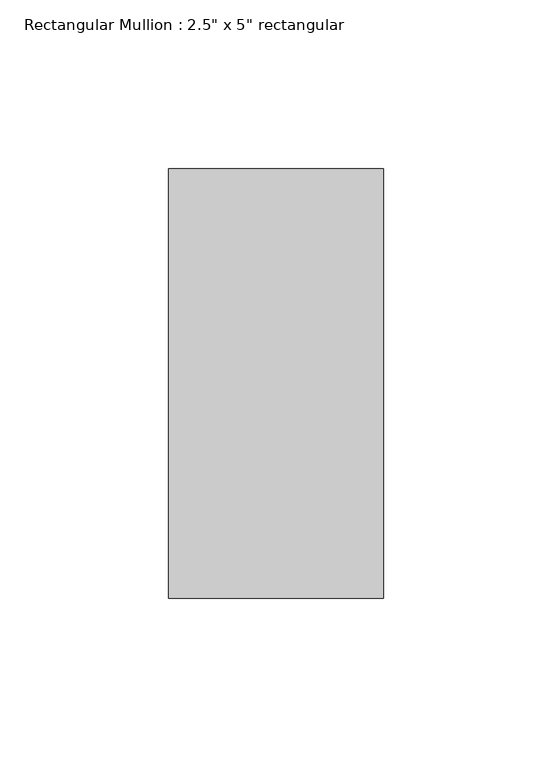
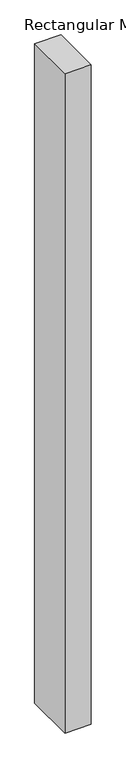
"""IFC4 building model written with IfcOpenShell, lengths in millimetres: member geometry."""

from ifc_helpers import new_model, si_unit, frame, origin, place, context, project, spatial, polyline, outline, extrude, source, transform, mapped, element, save


def member_26ad134e(model_context):
    return source(origin(), model_context, "Body", "SweptSolid", [
        extrude(outline(polyline([(0.0, 63.5), (0.0, -63.5), (-63.5, -63.5), (-63.5, 63.5), (0.0, 63.5)])), frame((0.0, 0.0, -1693.6943888), z_axis=(0.0, 0.0, 1.0), x_axis=(1.0, 0.0, 0.0)), (0.0, 0.0, 1.0), 1693.6943888),
    ])


if __name__ == "__main__":
    model = new_model("IFC4")
    model_context = context("Model", 3, world=origin())
    ifc_project = project(units=[si_unit("LENGTHUNIT", "METRE", prefix="MILLI")], contexts=[model_context])
    site = spatial("IfcSite", under=ifc_project)
    building = spatial("IfcBuilding", under=site)
    placement = place(None, origin())
    member_shape = member_26ad134e(model_context)
    element("IfcMember", 1, ObjectType="Rectangular Mullion : 2.5\" x 5\" rectangular", at=placement, inside=building, context=model_context, shape_type="MappedRepresentation", body=[
        mapped(member_shape, transform((0.0, 0.0, 0.0), x_axis=(1.0, 0.0, 0.0), y_axis=(0.0, 1.0, 0.0), z_axis=(0.0, 0.0, 1.0))),
    ])
    save(model, "model.ifc")

# Revit data of these elements
# Type "Rectangular Mullion : 2.5\" x 5\" rectangular"
#   built-in parameter 1007304 = 0.416667 (stored number, unit not read)
#   built-in parameter 1007301 = 0.104167 (stored number, unit not read)
#   built-in parameter 1007300 = 0.104167 (stored number, unit not read)
# Element 1 (IfcMember, "Rectangular Mullion : 2.5\" x 5\" rectangular")
#   Materials on its faces: "Aluminum"
# Materials
#   "Aluminum": class "Metal", colour RGB 247 247 247, transparency 0, Description = "Aluminum 6061", Cost = 0
